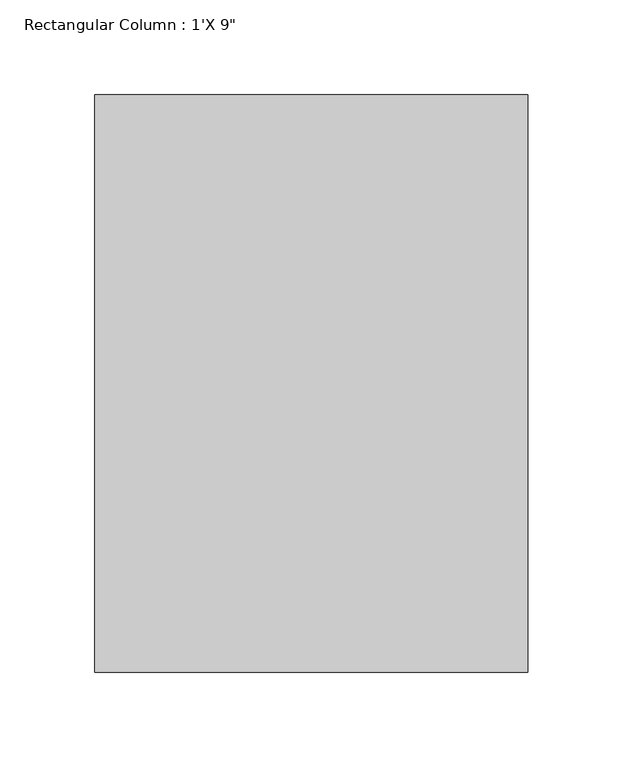
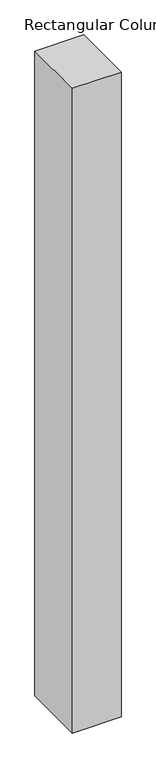
"""IFC4 building model written with IfcOpenShell, lengths in millimetres: column geometry."""

from ifc_helpers import new_model, si_unit, origin, origin_with_axes, place, context, project, spatial, polyline, outline, extrude, source, transform, mapped, element, save


def column_f87144f2(model_context):
    return source(origin(), model_context, "Body", "SweptSolid", [
        extrude(outline(polyline([(114.3, 152.4), (114.3, -152.4), (-114.3, -152.4), (-114.3, 152.4), (114.3, 152.4)])), origin_with_axes(), (0.0, 0.0, 1.0), 3200.4),
    ])


if __name__ == "__main__":
    model = new_model("IFC4")
    model_context = context("Model", 3, world=origin())
    ifc_project = project(units=[si_unit("LENGTHUNIT", "METRE", prefix="MILLI")], contexts=[model_context])
    site = spatial("IfcSite", under=ifc_project)
    building = spatial("IfcBuilding", under=site)
    placement = place(None, origin())
    column_shape = column_f87144f2(model_context)
    element("IfcColumn", 1, ObjectType="Rectangular Column : 1'X 9\"", at=placement, inside=building, context=model_context, shape_type="MappedRepresentation", body=[
        mapped(column_shape, transform((0.0, 0.0, 0.0), x_axis=(1.0, 0.0, 0.0), y_axis=(0.0, 1.0, 0.0), z_axis=(0.0, 0.0, 1.0))),
    ])
    save(model, "model.ifc")

# Revit data of these elements
# Type "Rectangular Column : 1'X 9\""
#   Assembly Code = "B1010200"
#   Depth = 1' - 0"
#   Offset Base = 0' - 0"
#   Offset Top = 0' - 0"
#   Width = 0' - 9"
#   Material = none
